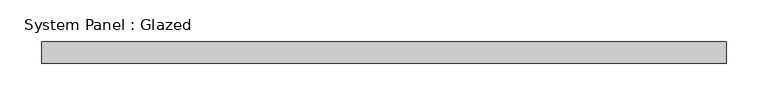
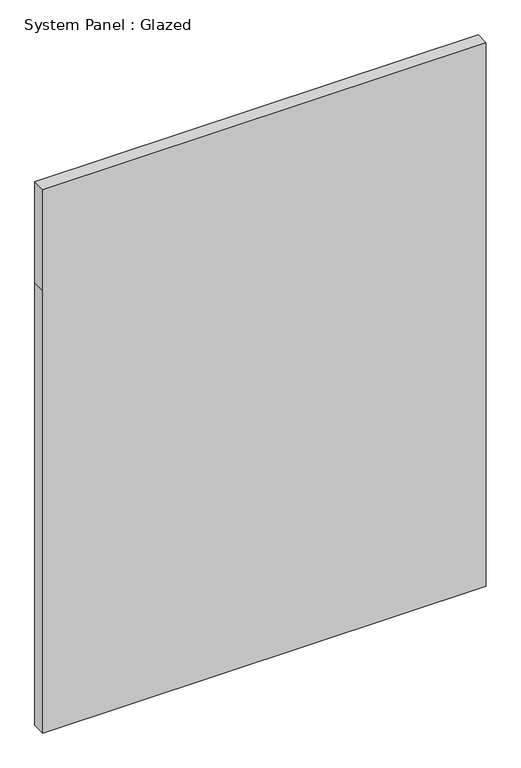
"""IFC4 building model written with IfcOpenShell, lengths in millimetres: plate geometry, System Panel : Glazed."""

from ifc_helpers import new_model, si_unit, frame, origin, place, context, project, spatial, polyline, outline, extrude, source, transform, mapped, element, save


def system_panel_glazed_48fb4df7(model_context):
    return source(origin(), model_context, "Body", "SweptSolid", [
        extrude(outline(polyline([(0.0, -409.575), (0.0, 409.575), (863.8653615, 409.575), (1060.7153615, 409.575), (1060.7153615, -409.575), (863.8653615, -409.575), (0.0, -409.575)])), frame((0.0, 19.05, 0.0), z_axis=(0.0, 1.0, 0.0), x_axis=(0.0, 0.0, 1.0)), (0.0, 0.0, 1.0), 25.4),
    ])


if __name__ == "__main__":
    model = new_model("IFC4")
    model_context = context("Model", 3, world=origin())
    ifc_project = project(units=[si_unit("LENGTHUNIT", "METRE", prefix="MILLI")], contexts=[model_context])
    site = spatial("IfcSite", under=ifc_project)
    building = spatial("IfcBuilding", under=site)
    placement = place(None, origin())
    system_panel_glazed_shape = system_panel_glazed_48fb4df7(model_context)
    element("IfcPlate", 1, ObjectType="System Panel : Glazed", at=placement, inside=building, context=model_context, shape_type="MappedRepresentation", body=[
        mapped(system_panel_glazed_shape, transform((0.0, 0.0, 0.0), x_axis=(1.0, 0.0, 0.0), y_axis=(0.0, 1.0, 0.0), z_axis=(0.0, 0.0, 1.0))),
    ])
    save(model, "model.ifc")

# Revit data of these elements
# Type "System Panel : Glazed"
#   Construction Type Id = "GSP4R"
#   Analytic Construction = "1/8 in Pilkington single glazing"
#   Visual Light Transmittance = 0.9
#   Solar Heat Gain Coefficient = 0.86
#   Heat Transfer Coefficient (U) = 1.18115 BTU/(h·ft²·°F)
#   Define Thermal Properties by = 1
# Element 1 (IfcPlate, "System Panel : Glazed")
#   Materials on its faces: "Glass"
# Materials
#   "Glass": class "Glass", colour RGB 0 128 192, transparency 0.75, Description = "Soda Lime Glass", Cost = 0
